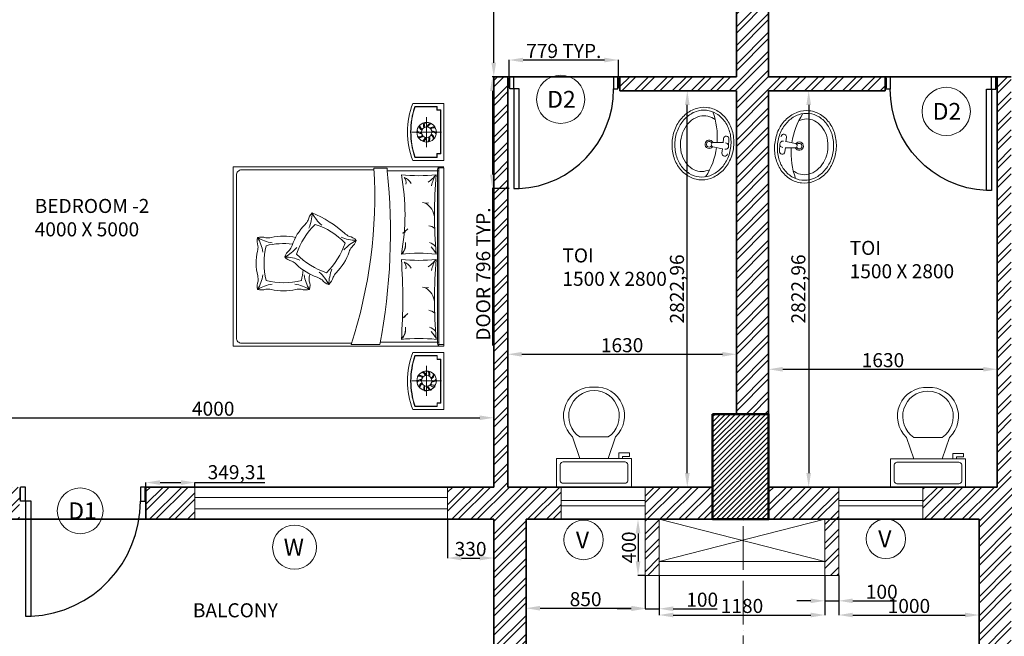
# Model space of a CAD drawing. Units: millimetres. Extents: x -3326 to 29338, y -16792 to 6002.
# Tile 3 of 21: x 233 to 7252, y -12098 to -7704. Entities that reach past the tile are written whole.
import ezdxf

# ---------------------------------------------------------------- set-up
doc = ezdxf.new("R2010")
doc.units = ezdxf.units.MM
doc.header["$PDMODE"] = 35
doc.header["$PDSIZE"] = 5
doc.linetypes.add('ACAD_ISO04W100', pattern=[30, 24, -3, 0, -3])
for name, color, linetype, lineweight in [('A-ANNO-DIMS', 2, 'Continuous', 13), ('A-ANNO-SYMB', 7, 'Continuous', 18), ('A-AREA-IDEN', 7, 'Continuous', 18), ('A-COLS', 1, 'Continuous', 50), ('A-COLS-PATT', 251, 'Continuous', 13), ('A-DOOR', 3, 'Continuous', 25), ('A-FLOR-FIXT', 9, 'Continuous', 18), ('A-FLOR-SHFT', 8, 'Continuous', 18), ('A-GLAZ', 4, 'Continuous', 18), ('A-GRID', 8, 'ACAD_ISO04W100', 13), ('A-WALL', 7, 'Continuous', 35), ('A-WALL-PATT', 252, 'Continuous', 13), ('furn', 28, 'Continuous', 18)]:
    doc.layers.add(name, color=color, linetype=linetype, lineweight=lineweight)
doc.styles.get("Standard").update_dxf_attribs({"font": 'arial.ttf'})
doc.dimstyles.new('ISO-25', dxfattribs={"dimtxt": 100, "dimasz": 100, "dimexe": 1.25, "dimexo": 0.625, "dimtad": 1, "dimtxsty": 'Standard', "dimcen": 2.5, "dimadec": 0, "dimazin": 0, "dimtfac": 1, "dimtmove": 0, "dimatfit": 3, "dimfxl": 1, "dimarcsym": 0})

# ---------------------------------------------------------------- blocks, each defined once
blk = doc.blocks.new('A$C0CE462CD')
for p, q in [((860, 100), (860, 0)), ((860, 0), (893.9, 0))]:
    blk.add_line(p, q)
for points in [[(860, 100), (860, 920), (818.4, 920), (818.4, 100)], [(0, 10), (6.1, 10), (6.1, 90), (0, 90)], [(893.9, 10), (900, 10), (900, 90), (893.9, 90)]]:
    blk.add_lwpolyline(points, close=True)
for points in [[(6.1, 0), (40, 0), (40, 100), (6.1, 100)], [(6.1, 100), (6.1, 0)], [(860, 100), (893.9, 100), (893.9, 0)]]:
    blk.add_lwpolyline(points)
blk.add_arc((859.1, 101.9), 819.1, 92.8508, 180.13091)
blk = doc.blocks.new('*U5')
for p, q in [((9.5, -6), (9.5, -2)), ((-8, -8.5), (-8, -8)), ((-7, -8), (-7, -9.5)), ((-4, -8), (-6, -14)), ((4, -8), (6, -14)), ((-10, -8.5), (-8, -8.5)), ((-10, -9.5), (-10, -8.5)), ((-7, -9.5), (-10, -9.5)), ((4, -14), (-4, -14))]:
    blk.add_line(p, q)
blk.add_lwpolyline([(10.5, -8), (10.5, 0), (-10.5, 0), (-10.5, -8)], close=True)
for points in [[(-9.5, -2), (-9.5, -6)], [(8.5, -1), (-8.5, -1)], [(-8.5, -7), (8.5, -7)]]:
    blk.add_lwpolyline(points)
for centre, radius, start, end in [((-8.625, -1.875), 0.8839, 81.8699, 188.1301), ((8.625, -1.875), 0.8839, 351.8699, 98.1301), ((-8.625, -6.125), 0.8839, 171.869898, 278.1301), ((8.625, -6.125), 0.8839, 261.8699, 8.1301), ((-0.4772, -19.9188), 8.0953, 133.01722, 273.38), ((0.0374, -19.8731), 7.127, 124.50543, 269.7), ((-0.0373, -19.8731), 7.127, 270.3, 55.4946), ((0.4773, -19.9188), 8.0953, 266.62, 46.9828)]:
    blk.add_arc(centre, radius, start, end)
blk = doc.blocks.new('A$C6B943AC5')
for p, q in [((0.207, 0.401), (0.2589, 0.4042)), ((0.2071, 0.362), (0.2386, 0.3621)), ((0.2361, 0.3625), (0.2439, 0.2926)), ((0.2809, 0.3627), (0.2736, 0.2927)), ((0.3111, 0.3624), (0.2796, 0.3623))]:
    blk.add_line(p, q)
for points in [[(0.518, 0.2209, -0.113917), (0.4993, 0.1385, -0.1036), (0.4427, 0.0651, -0.091717), (0.3606, 0.0176, -0.084781), (0.2598, 0, -0.084781), (0.1587, 0.0169, -0.091717), (0.0764, 0.0638, -0.1036), (0.0193, 0.1368, -0.113917), (0, 0.2191, -0.113917), (0.0187, 0.3015, -0.1036), (0.0753, 0.3749, -0.091717), (0.1574, 0.4224, -0.084781), (0.2582, 0.44, -0.084781), (0.3592, 0.4231, -0.091717), (0.4416, 0.3762, -0.1036), (0.4987, 0.3032, -0.113917)], [(0.498, 0.2208, -0.113917), (0.4813, 0.1472, -0.1036), (0.4297, 0.0803, -0.091717), (0.3539, 0.0364, -0.084781), (0.2597, 0.02, -0.084781), (0.1653, 0.0358, -0.091717), (0.0893, 0.0791, -0.1036), (0.0372, 0.1457, -0.113917), (0.02, 0.2192, -0.113917), (0.0367, 0.2928, -0.1036), (0.0883, 0.3597, -0.091717), (0.1641, 0.4036, -0.084781), (0.2583, 0.42, -0.084781), (0.3527, 0.4042, -0.091717), (0.4287, 0.3609, -0.1036), (0.4808, 0.2943, -0.113917)]]:
    blk.add_lwpolyline(points, format="xyb", close=True)
for points in [[(0.458, 0.2207, -0.113917), (0.4453, 0.1646, -0.1036), (0.4037, 0.1107, -0.091717), (0.3405, 0.0741, -0.084781), (0.2595, 0.06, -0.084781), (0.1785, 0.0736, -0.091717), (0.1151, 0.1097, -0.1036), (0.0731, 0.1633, -0.113917), (0.06, 0.2193, -0.113917), (0.0727, 0.2754, -0.020517), (0.0792, 0.2874, -0.091717)], [(0.4384, 0.2886, -0.020517), (0.4449, 0.2767, -0.113917), (0.458, 0.2207, -0.113917)]]:
    blk.add_lwpolyline(points, format="xyb")
for centre, radius, start, end in [((0.207, 0.3815), 0.0195, 90.19698, 270.19698), ((0.259, 0.3817), 0.0225, 354.08148, 186.31248), ((0.311, 0.3819), 0.0195, 270.19698, 90.19698), ((0.2604, -0.2004), 0.5204, 92.15427, 116.77617), ((0.2588, 0.265), 0.03, 119.152, 61.24195), ((0.2588, 0.265), 0.02, 116.58131, 63.81265), ((0.2587, 0.295), 0.015, 189.39225, 351.00171), ((0.2604, -0.2004), 0.5204, 63.61779, 88.23969)]:
    blk.add_arc(centre, radius, start, end)
blk = doc.blocks.new('*D61')
at = {"layer": 'A-ANNO-DIMS', "color": 0, "lineweight": -2, "transparency": 16777216}
for p, q in [((4692.3, -11664.6), (4692.3, -11902.5)), ((4792.3, -11664.6), (4792.3, -11902.5)), ((4592.3, -11901.3), (4492.3, -11901.3)), ((4692.3, -11901.3), (4792.3, -11901.3)), ((4892.3, -11901.3), (5204.7, -11901.3))]:
    blk.add_line(p, q, dxfattribs=at)
at = {"layer": 'A-ANNO-DIMS', "color": 0, "transparency": 16777216}
for points in [[(4592.3, -11884.6), (4592.3, -11918), (4692.3, -11901.3)], [(4892.3, -11884.6), (4892.3, -11918), (4792.3, -11901.3)]]:
    blk.add_solid(points, dxfattribs=at)
at = {"layer": 'Defpoints', "color": 0, "transparency": 16777216}
for p in [(4692.3, -11664), (4792.3, -11664), (4792.3, -11901.3)]:
    blk.add_point(p, dxfattribs=at)
at = {"layer": 'A-ANNO-DIMS', "color": 0, "transparency": 16777216, "insert": (5098.5, -11849.6), "char_height": 100, "attachment_point": 5}
blk.add_mtext('100', dxfattribs=at)
blk = doc.blocks.new('*D62')
at = {"layer": 'A-ANNO-DIMS', "color": 0, "lineweight": -2, "transparency": 16777216}
for p, q in [((5972.3, -11664.6), (5972.3, -11846)), ((6072.3, -11664.6), (6072.3, -11846)), ((5872.3, -11844.8), (5772.3, -11844.8)), ((5972.3, -11844.8), (6072.3, -11844.8)), ((6172.3, -11844.8), (6484.7, -11844.8))]:
    blk.add_line(p, q, dxfattribs=at)
at = {"layer": 'A-ANNO-DIMS', "color": 0, "transparency": 16777216}
for points in [[(5872.3, -11828.1), (5872.3, -11861.4), (5972.3, -11844.8)], [(6172.3, -11828.1), (6172.3, -11861.4), (6072.3, -11844.8)]]:
    blk.add_solid(points, dxfattribs=at)
at = {"layer": 'Defpoints', "color": 0, "transparency": 16777216}
for p in [(5972.3, -11664), (6072.3, -11664), (6072.3, -11844.8)]:
    blk.add_point(p, dxfattribs=at)
at = {"layer": 'A-ANNO-DIMS', "color": 0, "transparency": 16777216, "insert": (6378.5, -11793.1), "char_height": 100, "attachment_point": 5}
blk.add_mtext('100', dxfattribs=at)
blk = doc.blocks.new('*D63')
at = {"layer": 'A-ANNO-DIMS', "color": 0, "lineweight": -2, "transparency": 16777216}
for p, q in [((4792.3, -11664.6), (4792.3, -11947.2)), ((5972.3, -11664.6), (5972.3, -11947.2)), ((4892.3, -11945.9), (5872.3, -11945.9))]:
    blk.add_line(p, q, dxfattribs=at)
at = {"layer": 'A-ANNO-DIMS', "color": 0, "transparency": 16777216}
for points in [[(4892.3, -11929.2), (4892.3, -11962.6), (4792.3, -11945.9)], [(5872.3, -11929.2), (5872.3, -11962.6), (5972.3, -11945.9)]]:
    blk.add_solid(points, dxfattribs=at)
at = {"layer": 'Defpoints', "color": 0, "transparency": 16777216}
for p in [(4792.3, -11664), (5972.3, -11664), (5972.3, -11945.9)]:
    blk.add_point(p, dxfattribs=at)
at = {"layer": 'A-ANNO-DIMS', "color": 0, "transparency": 16777216, "insert": (5382.3, -11894.2), "char_height": 100, "attachment_point": 5}
blk.add_mtext('1180', dxfattribs=at)
blk = doc.blocks.new('*D64')
at = {"layer": 'A-ANNO-DIMS', "color": 0, "lineweight": -2, "transparency": 16777216}
for p, q in [((4692.3, -11744.2), (4692.3, -11898.8)), ((3842.3, -11797.8), (3842.3, -11898.8)), ((3942.3, -11897.5), (4592.3, -11897.5))]:
    blk.add_line(p, q, dxfattribs=at)
at = {"layer": 'A-ANNO-DIMS', "color": 0, "transparency": 16777216}
for points in [[(3942.3, -11880.9), (3942.3, -11914.2), (3842.3, -11897.5)], [(4592.3, -11880.9), (4592.3, -11914.2), (4692.3, -11897.5)]]:
    blk.add_solid(points, dxfattribs=at)
at = {"layer": 'Defpoints', "color": 0, "transparency": 16777216}
for p in [(4692.3, -11743.6), (3842.3, -11797.2), (4692.3, -11897.5)]:
    blk.add_point(p, dxfattribs=at)
at = {"layer": 'A-ANNO-DIMS', "color": 0, "transparency": 16777216, "insert": (4267.3, -11845.9), "char_height": 100, "attachment_point": 5}
blk.add_mtext('850', dxfattribs=at)
blk = doc.blocks.new('*D65')
at = {"layer": 'A-ANNO-DIMS', "color": 0, "lineweight": -2, "transparency": 16777216}
for p, q in [((6072.3, -11755.9), (6072.3, -11947.2)), ((7072.3, -11755.9), (7072.3, -11947.2)), ((6172.3, -11946), (6972.3, -11946))]:
    blk.add_line(p, q, dxfattribs=at)
at = {"layer": 'A-ANNO-DIMS', "color": 0, "transparency": 16777216}
for points in [[(6172.3, -11929.3), (6172.3, -11962.7), (6072.3, -11946)], [(6972.3, -11929.3), (6972.3, -11962.7), (7072.3, -11946)]]:
    blk.add_solid(points, dxfattribs=at)
at = {"layer": 'Defpoints', "color": 0, "transparency": 16777216}
for p in [(6072.3, -11755.3), (7072.3, -11755.3), (7072.3, -11946)]:
    blk.add_point(p, dxfattribs=at)
at = {"layer": 'A-ANNO-DIMS', "color": 0, "transparency": 16777216, "insert": (6572.3, -11894.3), "char_height": 100, "attachment_point": 5}
blk.add_mtext('1000', dxfattribs=at)
blk = doc.blocks.new('*D66')
at = {"layer": 'A-ANNO-DIMS', "color": 0, "lineweight": -2, "transparency": 16777216}
for p, q in [((4691.7, -11264), (4639.6, -11264)), ((4640.9, -11364), (4640.9, -11564)), ((4691.7, -11664), (4639.6, -11664))]:
    blk.add_line(p, q, dxfattribs=at)
at = {"layer": 'A-ANNO-DIMS', "color": 0, "transparency": 16777216}
for points in [[(4624.2, -11364), (4657.5, -11364), (4640.9, -11264)], [(4624.2, -11564), (4657.5, -11564), (4640.9, -11664)]]:
    blk.add_solid(points, dxfattribs=at)
at = {"layer": 'Defpoints', "color": 0, "transparency": 16777216}
for p in [(4692.3, -11264), (4640.9, -11664), (4692.3, -11664)]:
    blk.add_point(p, dxfattribs=at)
at = {"layer": 'A-ANNO-DIMS', "color": 0, "transparency": 16777216, "insert": (4589.2, -11464), "char_height": 100, "attachment_point": 5, "rotation": 90}
blk.add_mtext('400', dxfattribs=at)
blk = doc.blocks.new('*D68')
at = {"layer": 'A-ANNO-DIMS', "color": 0, "lineweight": -2, "transparency": 16777216}
for p, q in [((5572.3, -10194.1), (5572.3, -10193.5)), ((5672.3, -10194.8), (7102.3, -10194.8)), ((7202.3, -10194.1), (7202.3, -10193.5))]:
    blk.add_line(p, q, dxfattribs=at)
at = {"layer": 'A-ANNO-DIMS', "color": 0, "transparency": 16777216}
for points in [[(5672.3, -10178.1), (5672.3, -10211.4), (5572.3, -10194.8)], [(7102.3, -10178.1), (7102.3, -10211.4), (7202.3, -10194.8)]]:
    blk.add_solid(points, dxfattribs=at)
at = {"layer": 'Defpoints', "color": 0, "transparency": 16777216}
for p in [(5572.3, -10194.8), (7202.3, -10194.8), (7202.3, -10194.8)]:
    blk.add_point(p, dxfattribs=at)
at = {"layer": 'A-ANNO-DIMS', "color": 0, "transparency": 16777216, "insert": (6387.3, -10143), "char_height": 100, "attachment_point": 5}
blk.add_mtext('1630', dxfattribs=at)
blk = doc.blocks.new('*D69')
at = {"layer": 'A-ANNO-DIMS', "color": 0, "lineweight": -2, "transparency": 16777216}
for p, q in [((5572.9, -8211), (5858.8, -8211)), ((5857.6, -8311), (5857.6, -10934)), ((5572.9, -11034), (5858.8, -11034))]:
    blk.add_line(p, q, dxfattribs=at)
at = {"layer": 'A-ANNO-DIMS', "color": 0, "transparency": 16777216}
for points in [[(5840.9, -8311), (5874.2, -8311), (5857.6, -8211)], [(5840.9, -10934), (5874.2, -10934), (5857.6, -11034)]]:
    blk.add_solid(points, dxfattribs=at)
at = {"layer": 'Defpoints', "color": 0, "transparency": 16777216}
for p in [(5572.3, -8211), (5572.3, -11034), (5857.6, -11034)]:
    blk.add_point(p, dxfattribs=at)
at = {"layer": 'A-ANNO-DIMS', "color": 0, "transparency": 16777216, "insert": (5796.8, -9622.5), "char_height": 100, "attachment_point": 5, "rotation": 90}
blk.add_mtext('2822,96', dxfattribs=at)
blk = doc.blocks.new('*D70')
at = {"layer": 'A-ANNO-DIMS', "color": 0, "lineweight": -2, "transparency": 16777216}
for p, q in [((3712.3, -10087.4), (3712.3, -10086.7)), ((3812.3, -10088), (5242.3, -10088)), ((5342.3, -10087.4), (5342.3, -10086.7))]:
    blk.add_line(p, q, dxfattribs=at)
at = {"layer": 'A-ANNO-DIMS', "color": 0, "transparency": 16777216}
for points in [[(3812.3, -10071.3), (3812.3, -10104.7), (3712.3, -10088)], [(5242.3, -10071.3), (5242.3, -10104.7), (5342.3, -10088)]]:
    blk.add_solid(points, dxfattribs=at)
at = {"layer": 'Defpoints', "color": 0, "transparency": 16777216}
for p in [(3712.3, -10088), (5342.3, -10088), (5342.3, -10088)]:
    blk.add_point(p, dxfattribs=at)
at = {"layer": 'A-ANNO-DIMS', "color": 0, "transparency": 16777216, "insert": (4527.3, -10036.3), "char_height": 100, "attachment_point": 5}
blk.add_mtext('1630', dxfattribs=at)
blk = doc.blocks.new('*D71')
at = {"layer": 'A-ANNO-DIMS', "color": 0, "lineweight": -2, "transparency": 16777216}
for p, q in [((4897.1, -8211), (4993.6, -8211)), ((4992.3, -10934), (4992.3, -8311)), ((4897.1, -11034), (4993.6, -11034))]:
    blk.add_line(p, q, dxfattribs=at)
at = {"layer": 'A-ANNO-DIMS', "color": 0, "transparency": 16777216}
for points in [[(4975.6, -8311), (5009, -8311), (4992.3, -8211)], [(4975.6, -10934), (5009, -10934), (4992.3, -11034)]]:
    blk.add_solid(points, dxfattribs=at)
at = {"layer": 'Defpoints', "color": 0, "transparency": 16777216}
for p in [(4896.5, -8211), (4992.3, -8211), (4896.5, -11034)]:
    blk.add_point(p, dxfattribs=at)
at = {"layer": 'A-ANNO-DIMS', "color": 0, "transparency": 16777216, "insert": (4931.6, -9622.5), "char_height": 100, "attachment_point": 5, "rotation": 90}
blk.add_mtext('2822,96', dxfattribs=at)
blk = doc.blocks.new('*D72')
at = {"layer": 'A-ANNO-DIMS', "color": 0, "lineweight": -2, "transparency": 16777216}
for p, q in [((3282.3, -11264.6), (3282.3, -11541.2)), ((3612.3, -11264.6), (3612.3, -11541.2)), ((3382.3, -11539.9), (3512.3, -11539.9))]:
    blk.add_line(p, q, dxfattribs=at)
at = {"layer": 'A-ANNO-DIMS', "color": 0, "transparency": 16777216}
for points in [[(3382.3, -11523.3), (3382.3, -11556.6), (3282.3, -11539.9)], [(3512.3, -11523.3), (3512.3, -11556.6), (3612.3, -11539.9)]]:
    blk.add_solid(points, dxfattribs=at)
at = {"layer": 'Defpoints', "color": 0, "transparency": 16777216}
for p in [(3282.3, -11264), (3612.3, -11264), (3612.3, -11539.9)]:
    blk.add_point(p, dxfattribs=at)
at = {"layer": 'A-ANNO-DIMS', "color": 0, "transparency": 16777216, "insert": (3447.3, -11488.2), "char_height": 100, "attachment_point": 5}
blk.add_mtext('330', dxfattribs=at)
blk = doc.blocks.new('*D75')
at = {"layer": 'A-ANNO-DIMS', "color": 0, "lineweight": -2, "transparency": 16777216}
for p, q in [((1133, -11034.2), (1133, -11000.8)), ((1233, -11002.1), (1382.3, -11002.1)), ((1482.3, -11033.3), (1482.3, -11000.8)), ((1482.3, -11002.1), (1979.3, -11002.1))]:
    blk.add_line(p, q, dxfattribs=at)
at = {"layer": 'A-ANNO-DIMS', "color": 0, "transparency": 16777216}
for points in [[(1233, -10985.4), (1233, -11018.7), (1133, -11002.1)], [(1382.3, -10985.4), (1382.3, -11018.7), (1482.3, -11002.1)]]:
    blk.add_solid(points, dxfattribs=at)
at = {"layer": 'Defpoints', "color": 0, "transparency": 16777216}
for p in [(1482.3, -11002.1), (1133, -11034.8), (1482.3, -11034)]:
    blk.add_point(p, dxfattribs=at)
at = {"layer": 'A-ANNO-DIMS', "color": 0, "transparency": 16777216, "insert": (1780.8, -10941.3), "char_height": 100, "attachment_point": 5}
blk.add_mtext('349,31', dxfattribs=at)
blk = doc.blocks.new('*D76')
at = {"layer": 'A-ANNO-DIMS', "color": 0, "lineweight": -2, "transparency": 16777216}
for p, q in [((-387.7, -10539.9), (-387.7, -10539.2)), ((-287.7, -10540.5), (3512.3, -10540.5)), ((3612.3, -10539.9), (3612.3, -10539.2))]:
    blk.add_line(p, q, dxfattribs=at)
at = {"layer": 'A-ANNO-DIMS', "color": 0, "transparency": 16777216}
for points in [[(-287.7, -10523.8), (-287.7, -10557.2), (-387.7, -10540.5)], [(3512.3, -10523.8), (3512.3, -10557.2), (3612.3, -10540.5)]]:
    blk.add_solid(points, dxfattribs=at)
at = {"layer": 'Defpoints', "color": 0, "transparency": 16777216}
for p in [(-387.7, -10540.5), (3612.3, -10540.5), (3612.3, -10540.5)]:
    blk.add_point(p, dxfattribs=at)
at = {"layer": 'A-ANNO-DIMS', "color": 0, "transparency": 16777216, "insert": (1612.3, -10488.8), "char_height": 100, "attachment_point": 5}
blk.add_mtext('4000', dxfattribs=at)
blk = doc.blocks.new('*D84')
at = {"layer": 'A-ANNO-DIMS', "color": 0, "lineweight": -2, "transparency": 16777216}
for p, q in [((3612.9, -6550.4), (3613.6, -6550.4)), ((3612.3, -8011), (3612.3, -6650.4)), ((3612.9, -8111), (3613.6, -8111))]:
    blk.add_line(p, q, dxfattribs=at)
at = {"layer": 'A-ANNO-DIMS', "color": 0, "transparency": 16777216}
for points in [[(3595.6, -6650.4), (3629, -6650.4), (3612.3, -6550.4)], [(3595.6, -8011), (3629, -8011), (3612.3, -8111)]]:
    blk.add_solid(points, dxfattribs=at)
at = {"layer": 'Defpoints', "color": 0, "transparency": 16777216}
for p in [(3612.3, -6550.4), (3612.3, -6550.4), (3612.3, -8111)]:
    blk.add_point(p, dxfattribs=at)
at = {"layer": 'A-ANNO-DIMS', "color": 0, "transparency": 16777216, "insert": (3551.6, -7330.7), "char_height": 100, "attachment_point": 5, "rotation": 90}
blk.add_mtext('1560,59', dxfattribs=at)
blk = doc.blocks.new('BED-WITH-NIGHTSTANDS')
for p, q in [((1378.9, 2083.2), (1378.9, 1869.8)), ((1272.3, 1976.5), (1485.6, 1976.5)), ((1466.8, 1702.3), (1097.4, 1702.3)), ((1455.8, 1708.6), (1455.8, 473.4)), ((1466.8, 480.5), (1049.3, 480.5)), ((1378.9, 98.8), (1378.9, 312.2)), ((1272.2, 205.5), (1485.6, 205.5))]:
    blk.add_line(p, q)
for points in [[(1279.5, 2182), (1501.4, 2182), (1501.4, 1775.2), (1279.5, 1775.2, -0.181818)], [(1097.4, 1719.6), (1097.4, 1702.3, -0.072944), (1045.8, 463.1), (840.6, 463.1, 0.092568), (1003.3, 1719.6)], [(1198.4, 1674.1, 0.058596), (1445.6, 1674.1, 0.036889), (1445.6, 1107.7, 0.052163), (1198.4, 1107.7, 0.093111)], [(1198.4, 1070.9, 0.058596), (1445.6, 1070.9, 0.036648), (1445.6, 500.8, 0.052163), (1198.4, 500.8, 0.036967)], [(1279.6, 0), (1501.5, 0), (1501.5, 406.8), (1279.6, 406.8, 0.181818)]]:
    blk.add_lwpolyline(points, format="xyb", close=True)
for points in [[(1454.8, 1797.4), (1295, 1797.4, -0.167087), (1295, 2159.8), (1454.8, 2159.8)], [(1454.8, 1799.6), (1296.6, 1799.6, -0.165559), (1296.6, 2157.6), (1454.8, 2157.6)], [(1003.9, 1708.6), (59.2, 1708.6, 0.414214), (22.2, 1671.6), (22.2, 510.4, 0.414214), (59.2, 473.4), (844.2, 473.4)], [(540, 1293.1, 0.091296), (562.8, 1401.4, 0.091296), (630.7, 1314.1, 0.091296)], [(583.2, 1320, 0.111006), (451.8, 1108.7, 0.119549), (665.6, 975.5, 0.107813), (797.5, 1186.1)], [(797.2, 1187.3, 0.121865), (583.2, 1319.9, 0.121865)], [(211.2, 1122.2, 0.091296), (173.3, 1226.2, 0.091296), (277.2, 1187.9, 0.091296)], [(768.3, 1228.3, 0.091296), (876.7, 1205.8, 0.091296), (789.5, 1137.6, 0.091296)], [(233.7, 1167.8, 0.111006), (234, 919, 0.119549), (485.8, 919, 0.033212), (497.4, 995.5)], [(475.6, 1065.1, 0.091296), (367.2, 1087.5, 0.091296), (454.4, 1155.8)], [(367.2, 1087.5, 0.159461), (418, 1058.9, -0.076283), (449.6, 1036.2, 0.115075), (598.7, 943.3, -0.076283), (633, 924.9, 0.159461), (681.1, 892)], [(703.9, 1000.2, 0.091296), (681.1, 892, 0.091296), (613.2, 979.3, 0.091296)], [(277.2, 894.6, 0.091296), (173.3, 856.3, 0.091296), (211.2, 960.3)], [(505.3, 960.3, 0.091296), (543.2, 856.3, 0.091296), (439.3, 894.6, 0.091296)], [(173.3, 856.3, 0.159461), (231.6, 858.9, -0.076283), (270.5, 856.3, 0.115075), (446, 856.3, -0.076283), (484.9, 858.9, 0.159461), (543.2, 856.3)], [(1454.9, 384.6), (1295.1, 384.6, 0.167087), (1295.1, 22.2), (1454.9, 22.2)], [(1454.9, 382.4), (1296.7, 382.4, 0.165559), (1296.7, 24.4), (1454.9, 24.4)]]:
    blk.add_lwpolyline(points, format="xyb")
for points in [[(1479.2, 2133.2), (1452.6, 2133.2), (1452.6, 2159.8)], [(1479.2, 2135.4), (1454.8, 2135.4), (1454.8, 2159.8)], [(1477, 2135.4), (1477, 1821.8)], [(1479.2, 2135.4), (1479.2, 1821.8)], [(1479.2, 1824), (1452.6, 1824), (1452.6, 1797.4)], [(1479.2, 1821.8), (1454.8, 1821.8), (1454.8, 1797.4)], [(1501.5, 1730.8), (0, 1730.8), (0, 451.2), (1501.5, 451.2)], [(1501.5, 463.1), (1466.8, 463.1), (1466.8, 1723.4), (1501.5, 1723.4), (1501.5, 451.2)], [(1479.3, 358), (1452.7, 358), (1452.7, 384.6)], [(1479.3, 360.2), (1454.9, 360.2), (1454.9, 384.6)], [(1477.1, 46.6), (1477.1, 360.2)], [(1479.3, 46.6), (1479.3, 360.2)], [(1479.3, 48.8), (1452.7, 48.8), (1452.7, 22.2)], [(1479.3, 46.6), (1454.9, 46.6), (1454.9, 22.2)]]:
    blk.add_lwpolyline(points)
for centre, radius in [((1378.9, 1976.5), 69.7), ((1378.9, 1976.5), 37.8), ((1378.9, 205.5), 69.7), ((1378.9, 205.5), 37.8)]:
    blk.add_circle(centre, radius)
for centre, radius, start, end in [((1400.9, 2024.2), 44.8, 154.17003, 200.48975), ((1396.5, 2024.6), 34.1, 142.30017, 202.53802), ((1424.8, 2002.2), 44.8, 118.17003, 164.48975), ((1421.4, 2005.1), 34.1, 106.30017, 166.53802), ((1340.3, 2012.2), 44.8, 226.17003, 272.48975), ((1338.5, 2008.1), 34.1, 214.30017, 274.53802), ((1368.7, 2028), 44.8, 190.17003, 236.48975), ((1364.8, 2025.8), 34.1, 178.30017, 238.53802), ((1431.1, 1970.3), 44.8, 82.17003, 128.48975), ((1430.1, 1974.7), 34.1, 70.30017, 130.53802), ((1417.5, 1940.8), 44.8, 46.17003, 92.48975), ((1419.3, 1944.9), 34.1, 34.30017, 94.53802), ((1327.7, 1978.3), 34.1, 250.30017, 310.53802), ((1326.7, 1982.7), 44.8, 262.17003, 308.48975), ((1336.4, 1947.9), 34.1, 286.30017, 346.53802), ((1333.1, 1950.8), 44.8, 298.17003, 344.48975), ((1361.4, 1928.3), 34.1, 322.30017, 22.53802), ((1356.9, 1928.8), 44.8, 334.17003, 20.48975), ((1393, 1927.2), 34.1, 358.30017, 58.53802), ((1389.2, 1925), 44.8, 10.17003, 56.48975), ((1478, 1708.6), 22.2, 90, 180), ((1175.6, 1619.4), 56.2, 346.48229, 38.55627), ((1192.7, 1576.7), 82.2, 24.2916, 70.9896), ((1214.5, 1859.4), 296.3, 306.49353, 321.27919), ((1652.3, 1542.6), 244.9, 147.53791, 167.5233), ((1375.3, 1532.7), 61.4, 245.89274, 286.11919), ((1299.1, 1354.7), 137.1, 6.68493, 58.3182), ((419.7, 1408.4), 128.4, 315.77185, 333.2208), ((626.3, 1332.5), 93.8, 132.65224, 168.89294), ((256.3, 651.7), 810, 48.38179, 67.76439), ((785.6, 1046.2), 386.5, 135.13065, 161.38844), ((1208.9, 1279), 20.7, 263.75428, 347.21866), ((1026.5, 1507.4), 308.8, 306.20852, 315.08491), ((1377, 1216.1), 96.2, 51.81741, 79.89867), ((263.7, 1201.2), 93.8, 164.57915, 200.81985), ((198.5, 1135.9), 93.8, 69.36661, 105.60731), ((242.7, 1351.6), 128.4, 265.03874, 282.4877), ((358.2, 849.8), 386.5, 76.87111, 103.12889), ((884.1, 1348.9), 128.4, 225.58539, 243.03435), ((807.5, 1142.5), 93.8, 42.46578, 78.70648), ((789.7, 1230.6), 90.5, 307.29372, 344.09733), ((550.3, 1042.5), 386.5, 167.05756, 193.31535), ((48.2, 1156.4), 128.4, 347.69876, 5.14771), ((360.8, 659.2), 524.3, 83.19556, 104.02838), ((468.2, 1051.5), 107.3, 128.77541, 160.35713), ((298.1, 1211.9), 128.4, 323.29829, 340.74724), ((460, 1247.6), 386.5, 315.13065, 341.38844), ((947.4, 1081.9), 128.4, 143.29829, 160.74724), ((1127.7, 1179.9), 101.1, 314.40604, 6.83423), ((1163, 1161), 64, 303.63488, 0.84559), ((1363.4, 1094.5), 103.5, 40.53543, 70.35581), ((1276.2, 1030), 186.4, 24.64565, 44.15848), ((1214.5, 1256.2), 296.3, 306.49353, 321.27919), ((1652.3, 939.4), 244.9, 147.53791, 167.5233), ((1175.6, 1016.2), 56.2, 346.48229, 38.55627), ((1192.7, 973.5), 82.2, 24.2916, 70.9896), ((278.1, 879.2), 107.3, 160.70232, 192.28404), ((48.9, 925.3), 128.4, 355.2252, 12.67415), ((669.5, 927.3), 128.4, 167.69876, 185.14771), ((461.1, 884), 86.6, 341.39955, 21.57741), ((167.4, 1041.2), 386.5, 347.05756, 348.7033), ((626.1, 958.8), 86.6, 309.47264, 349.6505), ((825.9, 885.4), 128.4, 135.77185, 153.2208), ((1375.3, 929.5), 61.4, 245.89274, 286.11919), ((1299.1, 751.6), 137.1, 6.68493, 58.3182), ((1377, 612.9), 96.2, 51.81741, 79.89867), ((1208.9, 675.8), 20.7, 263.75428, 347.21866), ((1026.5, 904.2), 308.8, 306.20852, 315.08491), ((1127.7, 576.7), 101.1, 314.40604, 6.83423), ((1363.4, 491.3), 103.5, 40.53543, 70.35581), ((1163, 557.8), 64, 303.63488, 0.84559), ((1276.2, 426.8), 186.4, 24.64565, 44.15848), ((1478, 473.4), 22.2, 180, 270), ((1340.3, 169.8), 44.8, 87.51025, 133.82997), ((1327.7, 203.7), 34.1, 49.46198, 109.69983), ((1326.7, 199.3), 44.8, 51.51025, 97.82997), ((1336.4, 234.2), 34.1, 13.46198, 73.69983), ((1333, 231.2), 44.8, 15.51025, 61.82997), ((1361.4, 253.7), 34.1, 337.46198, 37.69983), ((1356.9, 253.2), 44.8, 339.51025, 25.82997), ((1393, 254.8), 34.1, 301.46198, 1.69983), ((1389.2, 257.1), 44.8, 303.51025, 349.82997), ((1419.3, 237.1), 34.1, 265.46198, 325.69983), ((1338.5, 173.9), 34.1, 85.46198, 145.69983), ((1368.6, 154), 44.8, 123.51025, 169.82997), ((1364.8, 156.2), 34.1, 121.46198, 181.69983), ((1402.8, 152.7), 44.8, 159.51025, 205.82997), ((1398.4, 152.3), 34.1, 157.46198, 217.69983), ((1426.7, 174.7), 44.8, 195.51025, 241.82997), ((1423.3, 171.8), 34.1, 193.46198, 253.69983), ((1433, 206.6), 44.8, 231.51025, 277.82997), ((1430.1, 207.3), 34.1, 229.46198, 289.69983), ((1417.5, 241.2), 44.8, 267.51025, 313.82997)]:
    blk.add_arc(centre, radius, start, end)
blk = doc.blocks.new('TAG-D1')
blk.add_circle((163.3, 163.3), 163.3)
at = {"insert": (78, 223.5), "char_height": 120, "attachment_point": 1}
blk.add_mtext_dynamic_manual_height_columns('D1', width=137.943, gutter_width=12.5, heights=[0], dxfattribs=at)
blk = doc.blocks.new('TAG-D2')
blk.add_circle((172, 172), 172)
at = {"insert": (75.7, 232.2), "char_height": 120, "attachment_point": 1}
blk.add_mtext_dynamic_manual_height_columns('D2', width=130.724, gutter_width=12.5, heights=[0], dxfattribs=at)
blk = doc.blocks.new('TAG-V')
blk.add_circle((140.7, 140.7), 140.7)
at = {"insert": (85.8, 200.7), "char_height": 120, "attachment_point": 1}
blk.add_mtext_dynamic_manual_height_columns('V', width=129.836, gutter_width=12.5, heights=[0], dxfattribs=at)
blk = doc.blocks.new('TAG-W')
blk.add_circle((156.8, 156.8), 156.8)
at = {"insert": (79.7, 216.8), "char_height": 120, "attachment_point": 1}
blk.add_mtext_dynamic_manual_height_columns('W', width=376.575, gutter_width=12.5, heights=[0], dxfattribs=at)
blk = doc.blocks.new('GLAZ-1800x80')
for p, q in [((0, 80), (1800, 80)), ((0, 0), (1800, 0))]:
    blk.add_line(p, q)
blk = doc.blocks.new('GLAZ-600x40')
for p, q in [((600, 40), (0, 40)), ((600, 0), (0, 0))]:
    blk.add_line(p, q)
blk = doc.blocks.new('*D191')
at = {"layer": 'A-ANNO-DIMS', "color": 0, "lineweight": -2, "transparency": 16777216}
for p, q in [((3721.4, -8111), (3601.3, -8111)), ((3602.6, -8211), (3602.6, -8807.4)), ((3721.4, -8907.4), (3601.3, -8907.4)), ((3602.6, -8907.4), (3602.6, -10026.1))]:
    blk.add_line(p, q, dxfattribs=at)
at = {"layer": 'A-ANNO-DIMS', "color": 0, "transparency": 16777216}
for points in [[(3585.9, -8211), (3619.2, -8211), (3602.6, -8111)], [(3585.9, -8807.4), (3619.2, -8807.4), (3602.6, -8907.4)]]:
    blk.add_solid(points, dxfattribs=at)
at = {"layer": 'Defpoints', "color": 0, "transparency": 16777216}
for p in [(3722, -8111), (3602.6, -8907.4), (3722, -8907.4)]:
    blk.add_point(p, dxfattribs=at)
at = {"layer": 'A-ANNO-DIMS', "color": 0, "transparency": 16777216, "insert": (3550.2, -9516.7), "char_height": 100, "attachment_point": 5, "rotation": 90}
blk.add_mtext('DOOR 796 TYP.', dxfattribs=at)
blk = doc.blocks.new('*D192')
at = {"layer": 'A-ANNO-DIMS', "color": 0, "lineweight": -2, "transparency": 16777216}
for p, q in [((3722, -8110.4), (3722, -7990.3)), ((4401.2, -7991.5), (3822, -7991.5)), ((4501.2, -8110.4), (4501.2, -7990.3))]:
    blk.add_line(p, q, dxfattribs=at)
at = {"layer": 'A-ANNO-DIMS', "color": 0, "transparency": 16777216}
for points in [[(3822, -7974.9), (3822, -8008.2), (3722, -7991.5)], [(4401.2, -7974.9), (4401.2, -8008.2), (4501.2, -7991.5)]]:
    blk.add_solid(points, dxfattribs=at)
at = {"layer": 'Defpoints', "color": 0, "transparency": 16777216}
for p in [(3722, -7991.5), (3722, -8111), (4501.2, -8111)]:
    blk.add_point(p, dxfattribs=at)
at = {"layer": 'A-ANNO-DIMS', "color": 0, "transparency": 16777216, "insert": (4111.6, -7939.8), "char_height": 100, "attachment_point": 5}
blk.add_mtext('779 TYP.', dxfattribs=at)

msp = doc.modelspace()

# ---------------------------------------------------------------- hatches: boundary and pattern name
at = {"layer": 'A-COLS-PATT'}
h = msp.add_hatch(dxfattribs=at)
h.set_pattern_fill('ANSI31', color=256, scale=8)
h.set_pattern_definition([(45, (-36866.33, -344.415), (-17.960512, 17.960512), [])])
h.paths.add_polyline_path([(5572.301, -10513.952), (5172.301, -10513.952), (5172.301, -11263.952), (5572.301, -11263.952)])
at = {"layer": 'A-WALL-PATT'}
h = msp.add_hatch(dxfattribs=at)
h.set_pattern_fill('ANSI32', color=256, scale=10)
h.set_pattern_definition([(45, (-10476.65, 1e-12), (-67.35192, 67.35192), []), (45, (-10431.74, 1e-12), (-67.35192, 67.35192), [])])
h.paths.add_polyline_path([(7302.301, -11263.952), (7902.301, -11263.952), (7902.301, -11033.952), (7302.301, -11033.952), (7302.301, -8110.991), (7202.301, -8110.991), (7202.301, -11033.952), (6672.301, -11033.952), (6672.301, -11263.952), (7072.301, -11263.952), (7072.301, -12763.952), (7302.301, -12763.952)])
h.paths.add_polyline_path([(9152.301, -11033.952), (8802.301, -11033.952), (8802.301, -11044.19), (8802.545, -11044.19), (8802.545, -11124.19), (8802.301, -11263.952), (9152.301, -11263.952)])
h.paths.add_polyline_path([(3712.301, -8110.991), (3612.301, -8110.991), (3612.301, -11033.952), (3282.301, -11033.952), (3282.301, -11263.952), (3612.301, -11263.952), (3612.301, -12763.952), (3842.301, -12763.952), (3842.301, -11263.952), (4092.301, -11263.952), (4092.301, -11033.952), (3842.301, -11033.952), (3712.301, -11033.952)])
h.paths.add_polyline_path([(5172.301, -11033.952), (4692.301, -11033.952), (4692.301, -11263.952), (5172.301, -11263.952)])
h.paths.add_polyline_path([(6072.301, -11033.952), (5572.301, -11033.952), (5572.301, -11263.952), (6072.301, -11263.952)])
h.paths.add_polyline_path([(6072.301, -11263.952), (5972.301, -11263.952), (5972.301, -11663.952), (6072.301, -11663.952)])
h.paths.add_polyline_path([(4792.301, -11263.952), (4692.301, -11263.952), (4692.301, -11663.952), (4792.301, -11663.952)])
h.paths.add_polyline_path([(6402.301, -8110.991), (6272.301, -8110.991), (5572.301, -8110.991), (5572.301, -7200.401), (5342.301, -7200.401), (5342.301, -8110.991), (4642.301, -8110.991), (4512.301, -8110.991), (4512.301, -8210.991), (4642.301, -8210.991), (5342.301, -8210.991), (5342.301, -10513.952), (5572.301, -10513.952), (5572.301, -8210.991), (6272.301, -8210.991), (6402.301, -8210.991)])
h.paths.add_polyline_path([(232.301, -11033.952), (-217.699, -11033.952), (-217.699, -11263.952), (232.301, -11263.952)])
h.paths.add_polyline_path([(1482.301, -11033.952), (1132.301, -11033.952), (1132.301, -11044.8), (1132.987, -11044.8), (1132.987, -11124.8), (1132.301, -11263.952), (1482.301, -11263.952)])
h.paths.add_polyline_path([(-387.699, -11263.952), (-617.699, -11263.952), (-617.699, -12763.952), (-438.882, -12763.952), (-387.699, -12763.952)])
h.paths.add_polyline_path([(-387.699, -7150.401), (-215.519, -7150.401), (-215.519, -7050.401), (-617.699, -7050.401), (-617.699, -10763.952), (-387.699, -10763.952)])
h.paths.add_polyline_path([(1512.301, -5983.952), (1282.301, -5983.952), (1282.301, -6450.401), (-215.519, -6450.401), (-215.519, -6550.401), (4073.51, -6550.401), (4073.51, -6450.401), (1512.301, -6450.401)])
h.paths.add_polyline_path([(5773.51, -6450.401), (5573.51, -6450.401), (5573.51, -6550.401), (5773.51, -6550.401)])
h.paths.add_polyline_path([(5173.51, -6450.401), (4973.51, -6450.401), (4973.51, -6550.401), (5173.51, -6550.401)])
h.paths.add_polyline_path([(10982.301, -6450.401), (6673.51, -6450.401), (6673.51, -6550.401), (10982.301, -6550.401)])

# ---------------------------------------------------------------- linework, layer by layer
at = {"layer": 'A-COLS'}
msp.add_lwpolyline([(5172.301, -10513.952), (5572.301, -10513.952), (5572.301, -11263.952), (5172.301, -11263.952)], close=True, dxfattribs=at)
at = {"layer": 'A-FLOR-SHFT'}
for p, q in [((4692.301, -11263.952), (4692.301, -11663.952)), ((4792.301, -11663.952), (4792.301, -11263.952)), ((4792.301, -11563.952), (5972.301, -11263.952)), ((4792.301, -11263.952), (5972.301, -11563.952)), ((5972.301, -11663.952), (5972.301, -11263.952)), ((6072.301, -11263.952), (6072.301, -11663.952)), ((4792.301, -11563.952), (5972.301, -11563.952)), ((4692.301, -11663.952), (4792.301, -11663.952)), ((4792.301, -11663.952), (5972.301, -11663.952)), ((6072.301, -11663.952), (5972.301, -11663.952))]:
    msp.add_line(p, q, dxfattribs=at)
at = {"layer": 'A-GLAZ'}
for p, q in [((1482.301, -11033.952), (1482.301, -11263.952)), ((3282.301, -11033.952), (3282.301, -11263.952)), ((4092.301, -11263.952), (4092.301, -11033.952)), ((4692.301, -11263.952), (4692.301, -11033.952)), ((6072.301, -11263.952), (6072.301, -11033.952)), ((6672.301, -11263.952), (6672.301, -11033.952))]:
    msp.add_line(p, q, dxfattribs=at)
at = {"layer": 'A-GRID', "ltscale": 13}
msp.add_line((5389.966, -13184.889), (5389.966, -11255.956), dxfattribs=at)
at = {"layer": 'A-WALL'}
for p, q in [((5572.301, -6450.401), (5572.301, -8110.991)), ((5342.301, -7200.401), (5342.301, -8110.991)), ((3842.301, -8110.991), (3612.301, -8110.991)), ((3612.301, -8110.991), (3612.301, -11033.952)), ((3712.301, -11033.952), (3712.301, -8110.991)), ((4642.301, -8110.991), (3842.301, -8110.991)), ((4512.301, -8110.991), (4512.301, -8210.991)), ((5342.301, -8110.991), (4642.301, -8110.991)), ((6272.301, -8110.991), (5572.301, -8110.991)), ((6272.301, -8110.991), (7072.301, -8110.991)), ((6402.301, -8110.991), (6402.301, -8210.991)), ((7302.301, -8110.991), (7072.301, -8110.991)), ((7202.301, -11033.952), (7202.301, -8110.991)), ((4512.301, -8210.991), (4642.301, -8210.991)), ((5342.301, -8210.991), (4642.301, -8210.991)), ((5342.301, -8210.991), (5342.301, -10513.952)), ((6272.301, -8210.991), (5572.301, -8210.991)), ((5572.301, -8210.991), (5572.301, -11263.952)), ((6402.301, -8210.991), (6272.301, -8210.991)), ((3612.301, -11033.952), (1132.301, -11033.952)), ((1132.301, -11033.952), (1132.301, -11263.952)), ((3842.301, -11033.952), (3712.301, -11033.952)), ((5173.51, -11033.952), (3842.301, -11033.952)), ((7202.301, -11033.952), (5572.301, -11033.952)), ((3612.301, -11263.952), (-217.699, -11263.952)), ((3612.301, -11263.952), (3612.301, -12763.952)), ((7072.301, -11263.952), (3842.301, -11263.952)), ((3842.301, -11263.952), (3842.301, -12763.952)), ((7072.301, -11263.952), (7072.301, -12763.952))]:
    msp.add_line(p, q, dxfattribs=at)

# ---------------------------------------------------------------- block references
at = {"layer": 'A-ANNO-SYMB'}
for name, p in [('TAG-D2', (3917.423, -8443.612)), ('TAG-D2', (6666.12, -8529.64)), ('TAG-D1', (500.809, -11366.978)), ('TAG-V', (4112.019, -11551.925)), ('TAG-V', (6267.607, -11543.947)), ('TAG-W', (2035.385, -11619.541))]:
    msp.add_blockref(name, p, dxfattribs=at)
at = {"layer": 'A-DOOR', "rotation": 180}
for p, xscale, yscale, zscale in [((4501.154, -8110.991), 0.86568603647667, 0.86568603647667, 0.86568603647667), ((6403.802, -8110.991), -0.8815660776293341, 0.8815660776293341, 0.8815660776293341)]:
    msp.add_blockref('A$C0CE462CD', p, dxfattribs=dict(at, xscale=xscale, yscale=yscale, zscale=zscale))
msp.add_blockref('A$C0CE462CD', (1132.987, -11034.8), dxfattribs=at)
at = {"layer": 'A-FLOR-FIXT'}
for name, p, xscale, yscale, zscale, rotation in [('A$C6B943AC5', (4914.056, -8304.916), 999.9999999999998, 999.9999999999998, 999.9999999999998, 263.5597085968623), ('A$C6B943AC5', (6024.31, -8891.981), 999.9999999999998, 999.9999999999998, 999.9999999999998, 83.55970859686228), ('*U5', (4327.217, -11032.763), 25.4, 25.4, 25.4, 180), ('*U5', (6708.149, -11035.528), 25.4, 25.4, 25.4, 180)]:
    msp.add_blockref(name, p, dxfattribs=dict(at, xscale=xscale, yscale=yscale, zscale=zscale, rotation=rotation))
at = {"layer": 'A-GLAZ'}
for name, p in [('GLAZ-1800x80', (1482.301, -11188.952)), ('GLAZ-600x40', (4092.301, -11168.952)), ('GLAZ-600x40', (6072.301, -11168.952))]:
    msp.add_blockref(name, p, dxfattribs=at)
at = {"layer": 'furn'}
msp.add_blockref('BED-WITH-NIGHTSTANDS', (1755.13, -10482.5), dxfattribs=at)

# ---------------------------------------------------------------- texts
at = {"layer": 'A-AREA-IDEN', "char_height": 100, "attachment_point": 1}
for s, insert in [('BEDROOM -2\\P4000 X 5000', (339.541, -8981.172)), ('TOI\\P1500 X 2800', (4101.647, -9333.875)), ('TOI\\P1500 X 2800', (6149.695, -9279.858)), ('BALCONY', (1467.24, -11862.223))]:
    msp.add_mtext_dynamic_manual_height_columns(s, width=1168.90663, gutter_width=12.5, heights=[0], dxfattribs=dict(at, insert=insert))

# ---------------------------------------------------------------- dimensions: what is measured, and where the dimension line sits
at = {"layer": 'A-ANNO-DIMS'}
for base, p1, p2, picture, middle in [((3612.301, -6550.401), (3612.301, -8110.991), (3612.301, -6550.401), '*D84', (3551.58, -7330.696)), ((4992.301, -8210.991), (4896.451, -11033.952), (4896.451, -8210.991), '*D71', (4931.58, -9622.472)), ((5857.553, -11033.952), (5572.301, -8210.991), (5572.301, -11033.952), '*D69', (5796.832, -9622.472)), ((4640.855, -11663.952), (4692.301, -11263.952), (4692.301, -11663.952), '*D66', (4589.172, -11463.952))]:
    dim = msp.add_linear_dim(base=base, p1=p1, p2=p2, angle=90, dimstyle='ISO-25', override={"dimclrd": 0, "dimclre": 0, "dimclrt": 0}, dxfattribs=at)
    dim.commit()
    dim.dimension.update_dxf_attribs({"geometry": picture, "text_midpoint": middle})
for base, p1, p2, angle, text, picture, middle in [((3722.036, -7991.527), (4501.154, -8110.991), (3722.036, -8110.991), 180, '<> TYP.', '*D192', (4111.595, -7939.844)), ((3602.572, -8907.422), (3722.036, -8110.991), (3722.036, -8907.422), 270, 'DOOR <> TYP.', '*D191', (3550.207, -9516.744))]:
    dim = msp.add_linear_dim(base=base, p1=p1, p2=p2, angle=angle, text=text, dimstyle='ISO-25', override={"dimdec": 0, "dimlfac": 1, "dimrnd": 0, "dimzin": 0, "dimdsep": 46, "dimlunit": 2}, dxfattribs=at)
    dim.commit()
    dim.dimension.update_dxf_attribs({"geometry": picture, "text_midpoint": middle})
for base, p1, p2, picture, middle in [((5342.301, -10087.997), (3712.301, -10087.997), (5342.301, -10087.997), '*D70', (4527.301, -10036.281)), ((7202.301, -10194.765), (5572.301, -10194.765), (7202.301, -10194.765), '*D68', (6387.301, -10143.049)), ((3612.301, -10540.499), (-387.699, -10540.499), (3612.301, -10540.499), '*D76', (1612.301, -10488.817)), ((1482.301, -11002.064), (1132.987, -11034.8), (1482.301, -11033.952), '*D75', (1780.811, -10941.344)), ((3612.301, -11539.933), (3282.301, -11263.952), (3612.301, -11263.952), '*D72', (3447.301, -11488.217)), ((4792.301, -11901.284), (4692.301, -11663.952), (4792.301, -11663.952), '*D61', (5098.519, -11849.602)), ((5972.301, -11945.912), (4792.301, -11663.952), (5972.301, -11663.952), '*D63', (5382.301, -11894.23)), ((6072.301, -11844.756), (5972.301, -11663.952), (6072.301, -11663.952), '*D62', (6378.519, -11793.073)), ((4692.301, -11897.534), (3842.301, -11797.153), (4692.301, -11743.6), '*D64', (4267.301, -11845.852)), ((7072.301, -11945.988), (6072.301, -11755.291), (7072.301, -11755.291), '*D65', (6572.301, -11894.306))]:
    dim = msp.add_linear_dim(base=base, p1=p1, p2=p2, dimstyle='ISO-25', override={"dimclrd": 0, "dimclre": 0, "dimclrt": 0}, dxfattribs=at)
    dim.commit()
    dim.dimension.update_dxf_attribs({"geometry": picture, "text_midpoint": middle})

doc.saveas('drawing.dxf')
